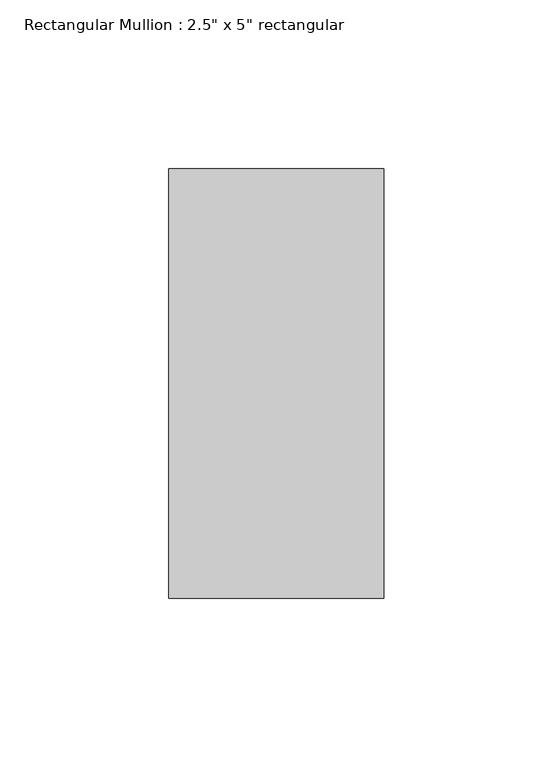
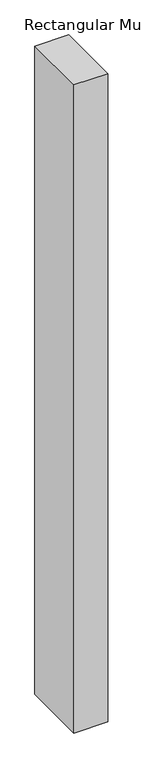
"""IFC4 building model written with IfcOpenShell, lengths in millimetres: member geometry."""

from ifc_helpers import new_model, si_unit, frame, origin, place, context, project, spatial, polyline, outline, extrude, source, transform, mapped, element, save


def member_6db20980(model_context):
    return source(origin(), model_context, "Body", "SweptSolid", [
        extrude(outline(polyline([(0.0, 63.5), (0.0, -63.5), (-63.5, -63.5), (-63.5, 63.5), (0.0, 63.5)])), frame((0.0, 0.0, -1288.0294817), z_axis=(0.0, 0.0, 1.0), x_axis=(1.0, 0.0, 0.0)), (0.0, 0.0, 1.0), 1288.0294817),
    ])


if __name__ == "__main__":
    model = new_model("IFC4")
    model_context = context("Model", 3, world=origin())
    ifc_project = project(units=[si_unit("LENGTHUNIT", "METRE", prefix="MILLI")], contexts=[model_context])
    site = spatial("IfcSite", under=ifc_project)
    building = spatial("IfcBuilding", under=site)
    placement = place(None, origin())
    member_shape = member_6db20980(model_context)
    element("IfcMember", 1, ObjectType="Rectangular Mullion : 2.5\" x 5\" rectangular", at=placement, inside=building, context=model_context, shape_type="MappedRepresentation", body=[
        mapped(member_shape, transform((0.0, 0.0, 0.0), x_axis=(1.0, 0.0, 0.0), y_axis=(0.0, 1.0, 0.0), z_axis=(0.0, 0.0, 1.0))),
    ])
    save(model, "model.ifc")

# Revit data of these elements
# Type "Rectangular Mullion : 2.5\" x 5\" rectangular"
#   built-in parameter 1007304 = 0.416667 (stored number, unit not read)
#   built-in parameter 1007301 = 0.104167 (stored number, unit not read)
#   built-in parameter 1007300 = 0.104167 (stored number, unit not read)
# Element 1 (IfcMember, "Rectangular Mullion : 2.5\" x 5\" rectangular")
#   Materials on its faces: "Aluminum"
# Materials
#   "Aluminum": class "Metal", colour RGB 247 247 247, transparency 0, Description = "Aluminum 6061", Cost = 0
